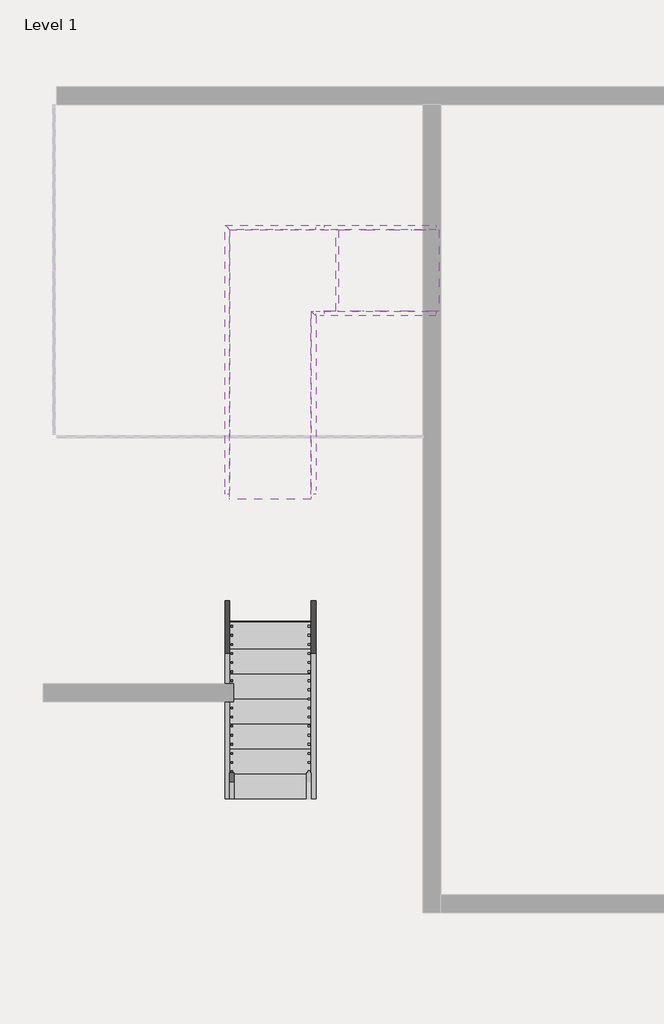
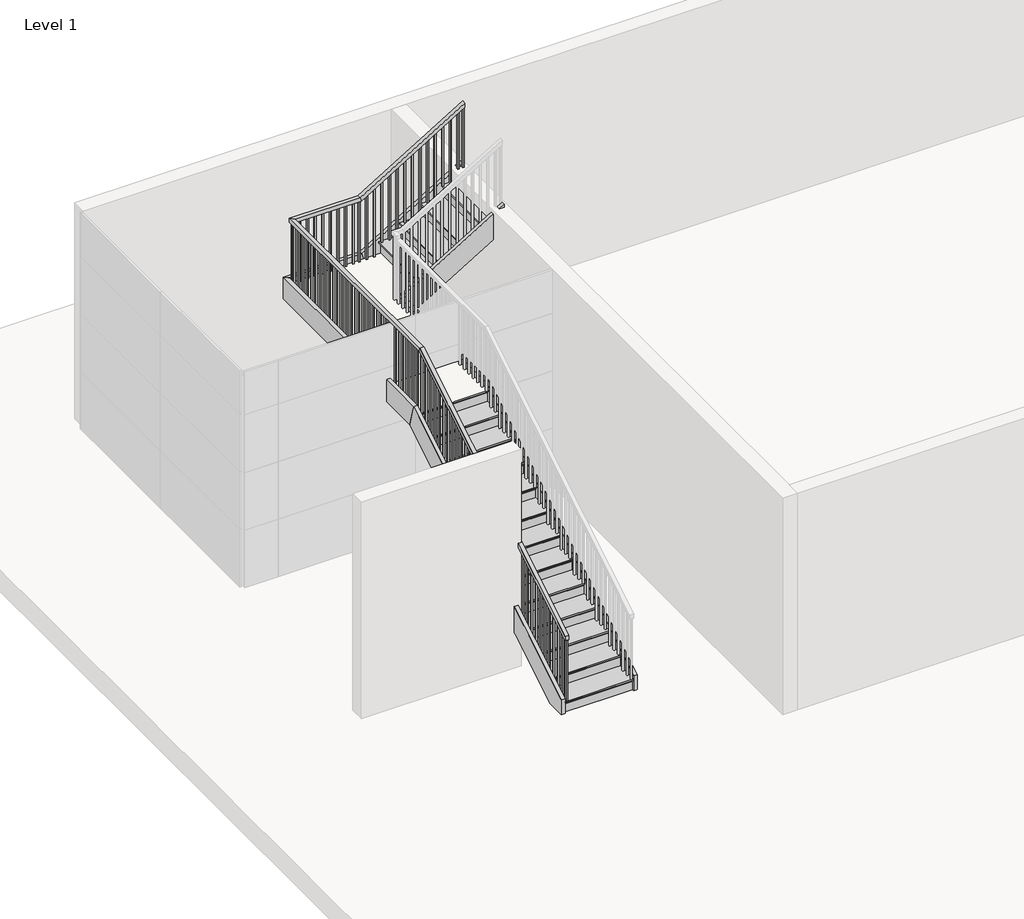
# One storey, part 2 of 2: 8 members, 2 stair flights, 1 railing, 1 slab.
"""IFC4 building model written with IfcOpenShell, lengths in millimetres."""

from ifc_helpers import new_model, si_unit, frame, origin, place, context, project, spatial, polyline, outline, extrude, faceted_brep, transform, mapped, element, save
from components import non_monolithic_landing_d9f9278d, stair_flight_de60d348, stair_flight_1517cfd2

model = new_model("IFC4")

# Units and contexts
model_context = context("Model", 3, world=origin())
ifc_project = project(units=[si_unit("LENGTHUNIT", "METRE", prefix="MILLI")], contexts=[model_context])

# Site, building, storey
site = spatial("IfcSite", under=ifc_project)
building = spatial("IfcBuilding", under=site)
storey = spatial("IfcBuildingStorey", under=building, Name="Level 1", Elevation=0.0)

# Members
placement = place(None, origin())
element("IfcMember", 1, ObjectType="Stringer - 2\" Width", at=placement, inside=storey, context=model_context, shape_type="SweptSolid", body=[
    extrude(outline(polyline([(1898.2635177, 0.0), (1898.2635177, 212.114512), (5306.204573, 2277.5333333), (5391.3590295, 1972.7333333), (2136.3490295, 0.0), (1898.2635177, 0.0)])), frame((-9085.0823175, 0.0, 0.0), z_axis=(1.0, 0.0, 0.0), x_axis=(0.0, 1.0, 0.0)), (0.0, 0.0, 1.0), 50.8),
])
element("IfcMember", 2, ObjectType="Stringer - 2\" Width", at=placement, inside=storey, context=model_context, shape_type="SweptSolid", body=[
    extrude(outline(polyline([(1898.2635177, 0.0), (1898.2635177, 212.114512), (5306.204573, 2277.5333333), (5391.3590295, 1972.7333333), (2136.3490295, 0.0), (1898.2635177, 0.0)])), frame((-8119.8823175, 0.0, 0.0), z_axis=(1.0, 0.0, 0.0), x_axis=(0.0, 1.0, 0.0)), (0.0, 0.0, 1.0), 50.8),
])
element("IfcMember", 3, ObjectType="Stringer - 2\" Width", at=placement, inside=storey, context=model_context, shape_type="SweptSolid", body=[
    extrude(outline(polyline([(2277.5333333, -8064.7412622), (1972.7333333, -7979.5868057), (2734.3724171, -6722.8823175), (3090.7811786, -6722.8823175), (2277.5333333, -8064.7412622)])), frame((0.0, 8266.605876, 0.0), z_axis=(0.0, 1.0, 0.0), x_axis=(0.0, 0.0, 1.0)), (0.0, 0.0, 1.0), 50.8),
])
element("IfcMember", 4, ObjectType="Stringer - 2\" Width", at=placement, inside=storey, context=model_context, shape_type="SweptSolid", body=[
    extrude(outline(polyline([(2277.5333333, -8064.7412622), (1972.7333333, -7979.5868057), (2734.3724171, -6722.8823175), (3090.7811786, -6722.8823175), (2277.5333333, -8064.7412622)])), frame((0.0, 7301.405876, 0.0), z_axis=(0.0, 1.0, 0.0), x_axis=(0.0, 0.0, 1.0)), (0.0, 0.0, 1.0), 50.8),
])
element("IfcMember", 5, ObjectType="Stringer - 2\" Width", at=placement, inside=storey, context=model_context, shape_type="Brep", body=[
    faceted_brep([(-8064.7412622, 8266.605876, 2277.5333333), (-8064.7412622, 8317.405876, 2277.5333333), (-9085.0823175, 8317.405876, 2277.5333333), (-9034.2823175, 8266.605876, 2277.5333333), (-7979.5868057, 8266.605876, 1972.7333333), (-9034.2823175, 8266.605876, 1972.7333333), (-7979.5868057, 8317.405876, 1972.7333333), (-9085.0823175, 8317.405876, 1972.7333333)], [[[0, 1, 2, 3]], [[4, 0, 3, 5]], [[6, 4, 5, 7]], [[1, 6, 7, 2]], [[1, 0, 4, 6]], [[2, 7, 5, 3]]]),
])
element("IfcMember", 6, ObjectType="Stringer - 2\" Width", at=placement, inside=storey, context=model_context, shape_type="Brep", body=[
    faceted_brep([(-9034.2823175, 8266.605876, 2277.5333333), (-9085.0823175, 8317.405876, 2277.5333333), (-9085.0823175, 5306.204573, 2277.5333333), (-9034.2823175, 5306.204573, 2277.5333333), (-9034.2823175, 8266.605876, 1972.7333333), (-9034.2823175, 5391.3590295, 1972.7333333), (-9085.0823175, 8317.405876, 1972.7333333), (-9085.0823175, 5391.3590295, 1972.7333333)], [[[0, 1, 2, 3]], [[4, 0, 3, 5]], [[6, 4, 5, 7]], [[1, 6, 7, 2]], [[1, 0, 4, 6]], [[2, 7, 5, 3]]]),
])
element("IfcMember", 7, ObjectType="Stringer - 2\" Width", at=placement, inside=storey, context=model_context, shape_type="Brep", body=[
    faceted_brep([(-8119.8823175, 5306.204573, 2277.5333333), (-8069.0823175, 5306.204573, 2277.5333333), (-8069.0823175, 7301.405876, 2277.5333333), (-8119.8823175, 7352.205876, 2277.5333333), (-8119.8823175, 5391.3590295, 1972.7333333), (-8119.8823175, 7352.205876, 1972.7333333), (-8069.0823175, 5391.3590295, 1972.7333333), (-8069.0823175, 7301.405876, 1972.7333333)], [[[0, 1, 2, 3]], [[4, 0, 3, 5]], [[6, 4, 5, 7]], [[1, 6, 7, 2]], [[1, 0, 4, 6]], [[2, 7, 5, 3]]]),
])
element("IfcMember", 8, ObjectType="Stringer - 2\" Width", at=placement, inside=storey, context=model_context, shape_type="Brep", body=[
    faceted_brep([(-8119.8823175, 7352.205876, 2277.5333333), (-8069.0823175, 7301.405876, 2277.5333333), (-8064.7412622, 7301.405876, 2277.5333333), (-8064.7412622, 7352.205876, 2277.5333333), (-8119.8823175, 7352.205876, 1972.7333333), (-7979.5868057, 7352.205876, 1972.7333333), (-8069.0823175, 7301.405876, 1972.7333333), (-7979.5868057, 7301.405876, 1972.7333333)], [[[0, 1, 2, 3]], [[4, 0, 3, 5]], [[6, 4, 5, 7]], [[1, 6, 7, 2]], [[1, 0, 4, 6]], [[2, 7, 5, 3]]]),
])

# Railing
element("IfcRailing", 9, ObjectType="Handrail - Rectangular", at=placement, inside=storey, context=model_context, shape_type="SolidModel", body=[
    faceted_brep([(-9034.2823175, 1898.2635177, 1083.7333333), (-9034.2823175, 1898.2635177, 1024.3318731), (-8983.4823175, 1898.2635177, 1024.3318731), (-8983.4823175, 1898.2635177, 1083.7333333), (-9034.2823175, 5251.0635177, 3115.7333333), (-9034.2823175, 5265.2559271, 3064.9333333), (-8983.4823175, 5265.2559271, 3064.9333333), (-8983.4823175, 5251.0635177, 3115.7333333), (-9034.2823175, 8266.605876, 3115.7333333), (-9034.2823175, 8266.605876, 3064.9333333), (-8983.4823175, 8215.805876, 3064.9333333), (-8983.4823175, 8215.805876, 3115.7333333), (-8119.8823175, 8266.605876, 3115.7333333), (-8105.6899081, 8266.605876, 3064.9333333), (-8105.6899081, 8215.805876, 3064.9333333), (-8119.8823175, 8215.805876, 3115.7333333), (-6722.8823175, 8266.605876, 3962.4), (-6722.8823175, 8215.805876, 3962.4), (-6722.8823175, 8215.805876, 3902.9985397), (-6722.8823175, 8266.605876, 3902.9985397)], [[[0, 1, 2, 3]], [[1, 0, 4, 5]], [[2, 1, 5, 6]], [[3, 2, 6, 7]], [[0, 3, 7, 4]], [[5, 4, 8, 9]], [[6, 5, 9, 10]], [[7, 6, 10, 11]], [[4, 7, 11, 8]], [[9, 8, 12, 13]], [[10, 9, 13, 14]], [[11, 10, 14, 15]], [[8, 11, 15, 12]], [[16, 17, 18, 19]], [[13, 12, 16, 19]], [[14, 13, 19, 18]], [[15, 14, 18, 17]], [[12, 15, 17, 16]]]),
    extrude(outline(polyline([(3851.0439943, -6808.6073175), (2878.6666667, -6808.6073175), (2878.6666667, -6789.5573175), (3862.5894488, -6789.5573175), (3851.0439943, -6808.6073175)])), frame((0.0, 8231.680876, 0.0), z_axis=(0.0, 1.0, 0.0), x_axis=(0.0, 0.0, 1.0)), (0.0, 0.0, 1.0), 19.05),
    extrude(outline(polyline([(3789.4682367, -6910.2073175), (2878.6666667, -6910.2073175), (2878.6666667, -6891.1573175), (3801.0136913, -6891.1573175), (3789.4682367, -6910.2073175)])), frame((0.0, 8231.680876, 0.0), z_axis=(0.0, 1.0, 0.0), x_axis=(0.0, 0.0, 1.0)), (0.0, 0.0, 1.0), 19.05),
    extrude(outline(polyline([(3727.8924791, -7011.8073175), (2878.6666667, -7011.8073175), (2878.6666667, -6992.7573175), (3739.4379337, -6992.7573175), (3727.8924791, -7011.8073175)])), frame((0.0, 8231.680876, 0.0), z_axis=(0.0, 1.0, 0.0), x_axis=(0.0, 0.0, 1.0)), (0.0, 0.0, 1.0), 19.05),
    extrude(outline(polyline([(3666.3167216, -7113.4073175), (2709.3333333, -7113.4073175), (2709.3333333, -7094.3573175), (3677.8621761, -7094.3573175), (3666.3167216, -7113.4073175)])), frame((0.0, 8231.680876, 0.0), z_axis=(0.0, 1.0, 0.0), x_axis=(0.0, 0.0, 1.0)), (0.0, 0.0, 1.0), 19.05),
    extrude(outline(polyline([(3604.740964, -7215.0073175), (2709.3333333, -7215.0073175), (2709.3333333, -7195.9573175), (3616.2864185, -7195.9573175), (3604.740964, -7215.0073175)])), frame((0.0, 8231.680876, 0.0), z_axis=(0.0, 1.0, 0.0), x_axis=(0.0, 0.0, 1.0)), (0.0, 0.0, 1.0), 19.05),
    extrude(outline(polyline([(3543.1652064, -7316.6073175), (2540.0, -7316.6073175), (2540.0, -7297.5573175), (3554.710661, -7297.5573175), (3543.1652064, -7316.6073175)])), frame((0.0, 8231.680876, 0.0), z_axis=(0.0, 1.0, 0.0), x_axis=(0.0, 0.0, 1.0)), (0.0, 0.0, 1.0), 19.05),
    extrude(outline(polyline([(3481.5894488, -7418.2073175), (2540.0, -7418.2073175), (2540.0, -7399.1573175), (3493.1349034, -7399.1573175), (3481.5894488, -7418.2073175)])), frame((0.0, 8231.680876, 0.0), z_axis=(0.0, 1.0, 0.0), x_axis=(0.0, 0.0, 1.0)), (0.0, 0.0, 1.0), 19.05),
    extrude(outline(polyline([(3420.0136913, -7519.8073175), (2540.0, -7519.8073175), (2540.0, -7500.7573175), (3431.5591458, -7500.7573175), (3420.0136913, -7519.8073175)])), frame((0.0, 8231.680876, 0.0), z_axis=(0.0, 1.0, 0.0), x_axis=(0.0, 0.0, 1.0)), (0.0, 0.0, 1.0), 19.05),
    extrude(outline(polyline([(3358.4379337, -7621.4073175), (2370.6666667, -7621.4073175), (2370.6666667, -7602.3573175), (3369.9833882, -7602.3573175), (3358.4379337, -7621.4073175)])), frame((0.0, 8231.680876, 0.0), z_axis=(0.0, 1.0, 0.0), x_axis=(0.0, 0.0, 1.0)), (0.0, 0.0, 1.0), 19.05),
    extrude(outline(polyline([(3296.8621761, -7723.0073175), (2370.6666667, -7723.0073175), (2370.6666667, -7703.9573175), (3308.4076307, -7703.9573175), (3296.8621761, -7723.0073175)])), frame((0.0, 8231.680876, 0.0), z_axis=(0.0, 1.0, 0.0), x_axis=(0.0, 0.0, 1.0)), (0.0, 0.0, 1.0), 19.05),
    extrude(outline(polyline([(3235.2864185, -7824.6073175), (2370.6666667, -7824.6073175), (2370.6666667, -7805.5573175), (3246.8318731, -7805.5573175), (3235.2864185, -7824.6073175)])), frame((0.0, 8231.680876, 0.0), z_axis=(0.0, 1.0, 0.0), x_axis=(0.0, 0.0, 1.0)), (0.0, 0.0, 1.0), 19.05),
    extrude(outline(polyline([(3173.710661, -7926.2073175), (2201.3333333, -7926.2073175), (2201.3333333, -7907.1573175), (3185.2561155, -7907.1573175), (3173.710661, -7926.2073175)])), frame((0.0, 8231.680876, 0.0), z_axis=(0.0, 1.0, 0.0), x_axis=(0.0, 0.0, 1.0)), (0.0, 0.0, 1.0), 19.05),
    extrude(outline(polyline([(3112.1349034, -8027.8073175), (2201.3333333, -8027.8073175), (2201.3333333, -8008.7573175), (3123.6803579, -8008.7573175), (3112.1349034, -8027.8073175)])), frame((0.0, 8231.680876, 0.0), z_axis=(0.0, 1.0, 0.0), x_axis=(0.0, 0.0, 1.0)), (0.0, 0.0, 1.0), 19.05),
    extrude(outline(polyline([(-8205.6073175, 8250.730876), (-8186.5573175, 8250.730876), (-8186.5573175, 8231.680876), (-8205.6073175, 8231.680876), (-8205.6073175, 8250.730876)])), frame((0.0, 0.0, 2201.3333333), z_axis=(0.0, 0.0, 1.0), x_axis=(1.0, 0.0, 0.0)), (0.0, 0.0, 1.0), 863.6),
    extrude(outline(polyline([(-8307.2073175, 8250.730876), (-8288.1573175, 8250.730876), (-8288.1573175, 8231.680876), (-8307.2073175, 8231.680876), (-8307.2073175, 8250.730876)])), frame((0.0, 0.0, 2201.3333333), z_axis=(0.0, 0.0, 1.0), x_axis=(1.0, 0.0, 0.0)), (0.0, 0.0, 1.0), 863.6),
    extrude(outline(polyline([(-8408.8073175, 8250.730876), (-8389.7573175, 8250.730876), (-8389.7573175, 8231.680876), (-8408.8073175, 8231.680876), (-8408.8073175, 8250.730876)])), frame((0.0, 0.0, 2201.3333333), z_axis=(0.0, 0.0, 1.0), x_axis=(1.0, 0.0, 0.0)), (0.0, 0.0, 1.0), 863.6),
    extrude(outline(polyline([(-8510.4073175, 8250.730876), (-8491.3573175, 8250.730876), (-8491.3573175, 8231.680876), (-8510.4073175, 8231.680876), (-8510.4073175, 8250.730876)])), frame((0.0, 0.0, 2201.3333333), z_axis=(0.0, 0.0, 1.0), x_axis=(1.0, 0.0, 0.0)), (0.0, 0.0, 1.0), 863.6),
    extrude(outline(polyline([(-8612.0073175, 8250.730876), (-8592.9573175, 8250.730876), (-8592.9573175, 8231.680876), (-8612.0073175, 8231.680876), (-8612.0073175, 8250.730876)])), frame((0.0, 0.0, 2201.3333333), z_axis=(0.0, 0.0, 1.0), x_axis=(1.0, 0.0, 0.0)), (0.0, 0.0, 1.0), 863.6),
    extrude(outline(polyline([(-8713.6073175, 8250.730876), (-8694.5573175, 8250.730876), (-8694.5573175, 8231.680876), (-8713.6073175, 8231.680876), (-8713.6073175, 8250.730876)])), frame((0.0, 0.0, 2201.3333333), z_axis=(0.0, 0.0, 1.0), x_axis=(1.0, 0.0, 0.0)), (0.0, 0.0, 1.0), 863.6),
    extrude(outline(polyline([(-8815.2073175, 8250.730876), (-8796.1573175, 8250.730876), (-8796.1573175, 8231.680876), (-8815.2073175, 8231.680876), (-8815.2073175, 8250.730876)])), frame((0.0, 0.0, 2201.3333333), z_axis=(0.0, 0.0, 1.0), x_axis=(1.0, 0.0, 0.0)), (0.0, 0.0, 1.0), 863.6),
    extrude(outline(polyline([(-8916.8073175, 8250.730876), (-8897.7573175, 8250.730876), (-8897.7573175, 8231.680876), (-8916.8073175, 8231.680876), (-8916.8073175, 8250.730876)])), frame((0.0, 0.0, 2201.3333333), z_axis=(0.0, 0.0, 1.0), x_axis=(1.0, 0.0, 0.0)), (0.0, 0.0, 1.0), 863.6),
    extrude(outline(polyline([(-9018.4073175, 8187.9385177), (-9018.4073175, 8206.9885177), (-8999.3573175, 8206.9885177), (-8999.3573175, 8187.9385177), (-9018.4073175, 8187.9385177)])), frame((0.0, 0.0, 2201.3333333), z_axis=(0.0, 0.0, 1.0), x_axis=(1.0, 0.0, 0.0)), (0.0, 0.0, 1.0), 863.6),
    extrude(outline(polyline([(-9018.4073175, 8086.3385177), (-9018.4073175, 8105.3885177), (-8999.3573175, 8105.3885177), (-8999.3573175, 8086.3385177), (-9018.4073175, 8086.3385177)])), frame((0.0, 0.0, 2201.3333333), z_axis=(0.0, 0.0, 1.0), x_axis=(1.0, 0.0, 0.0)), (0.0, 0.0, 1.0), 863.6),
    extrude(outline(polyline([(-9018.4073175, 7984.7385177), (-9018.4073175, 8003.7885177), (-8999.3573175, 8003.7885177), (-8999.3573175, 7984.7385177), (-9018.4073175, 7984.7385177)])), frame((0.0, 0.0, 2201.3333333), z_axis=(0.0, 0.0, 1.0), x_axis=(1.0, 0.0, 0.0)), (0.0, 0.0, 1.0), 863.6),
    extrude(outline(polyline([(-9018.4073175, 7883.1385177), (-9018.4073175, 7902.1885177), (-8999.3573175, 7902.1885177), (-8999.3573175, 7883.1385177), (-9018.4073175, 7883.1385177)])), frame((0.0, 0.0, 2201.3333333), z_axis=(0.0, 0.0, 1.0), x_axis=(1.0, 0.0, 0.0)), (0.0, 0.0, 1.0), 863.6),
    extrude(outline(polyline([(-9018.4073175, 7781.5385177), (-9018.4073175, 7800.5885177), (-8999.3573175, 7800.5885177), (-8999.3573175, 7781.5385177), (-9018.4073175, 7781.5385177)])), frame((0.0, 0.0, 2201.3333333), z_axis=(0.0, 0.0, 1.0), x_axis=(1.0, 0.0, 0.0)), (0.0, 0.0, 1.0), 863.6),
    extrude(outline(polyline([(-9018.4073175, 7679.9385177), (-9018.4073175, 7698.9885177), (-8999.3573175, 7698.9885177), (-8999.3573175, 7679.9385177), (-9018.4073175, 7679.9385177)])), frame((0.0, 0.0, 2201.3333333), z_axis=(0.0, 0.0, 1.0), x_axis=(1.0, 0.0, 0.0)), (0.0, 0.0, 1.0), 863.6),
    extrude(outline(polyline([(-9018.4073175, 7578.3385177), (-9018.4073175, 7597.3885177), (-8999.3573175, 7597.3885177), (-8999.3573175, 7578.3385177), (-9018.4073175, 7578.3385177)])), frame((0.0, 0.0, 2201.3333333), z_axis=(0.0, 0.0, 1.0), x_axis=(1.0, 0.0, 0.0)), (0.0, 0.0, 1.0), 863.6),
    extrude(outline(polyline([(-9018.4073175, 7476.7385177), (-9018.4073175, 7495.7885177), (-8999.3573175, 7495.7885177), (-8999.3573175, 7476.7385177), (-9018.4073175, 7476.7385177)])), frame((0.0, 0.0, 2201.3333333), z_axis=(0.0, 0.0, 1.0), x_axis=(1.0, 0.0, 0.0)), (0.0, 0.0, 1.0), 863.6),
    extrude(outline(polyline([(-9018.4073175, 7375.1385177), (-9018.4073175, 7394.1885177), (-8999.3573175, 7394.1885177), (-8999.3573175, 7375.1385177), (-9018.4073175, 7375.1385177)])), frame((0.0, 0.0, 2201.3333333), z_axis=(0.0, 0.0, 1.0), x_axis=(1.0, 0.0, 0.0)), (0.0, 0.0, 1.0), 863.6),
    extrude(outline(polyline([(-9018.4073175, 7273.5385177), (-9018.4073175, 7292.5885177), (-8999.3573175, 7292.5885177), (-8999.3573175, 7273.5385177), (-9018.4073175, 7273.5385177)])), frame((0.0, 0.0, 2201.3333333), z_axis=(0.0, 0.0, 1.0), x_axis=(1.0, 0.0, 0.0)), (0.0, 0.0, 1.0), 863.6),
    extrude(outline(polyline([(-9018.4073175, 7171.9385177), (-9018.4073175, 7190.9885177), (-8999.3573175, 7190.9885177), (-8999.3573175, 7171.9385177), (-9018.4073175, 7171.9385177)])), frame((0.0, 0.0, 2201.3333333), z_axis=(0.0, 0.0, 1.0), x_axis=(1.0, 0.0, 0.0)), (0.0, 0.0, 1.0), 863.6),
    extrude(outline(polyline([(-9018.4073175, 7070.3385177), (-9018.4073175, 7089.3885177), (-8999.3573175, 7089.3885177), (-8999.3573175, 7070.3385177), (-9018.4073175, 7070.3385177)])), frame((0.0, 0.0, 2201.3333333), z_axis=(0.0, 0.0, 1.0), x_axis=(1.0, 0.0, 0.0)), (0.0, 0.0, 1.0), 863.6),
    extrude(outline(polyline([(-9018.4073175, 6968.7385177), (-9018.4073175, 6987.7885177), (-8999.3573175, 6987.7885177), (-8999.3573175, 6968.7385177), (-9018.4073175, 6968.7385177)])), frame((0.0, 0.0, 2201.3333333), z_axis=(0.0, 0.0, 1.0), x_axis=(1.0, 0.0, 0.0)), (0.0, 0.0, 1.0), 863.6),
    extrude(outline(polyline([(-9018.4073175, 6867.1385177), (-9018.4073175, 6886.1885177), (-8999.3573175, 6886.1885177), (-8999.3573175, 6867.1385177), (-9018.4073175, 6867.1385177)])), frame((0.0, 0.0, 2201.3333333), z_axis=(0.0, 0.0, 1.0), x_axis=(1.0, 0.0, 0.0)), (0.0, 0.0, 1.0), 863.6),
    extrude(outline(polyline([(-9018.4073175, 6765.5385177), (-9018.4073175, 6784.5885177), (-8999.3573175, 6784.5885177), (-8999.3573175, 6765.5385177), (-9018.4073175, 6765.5385177)])), frame((0.0, 0.0, 2201.3333333), z_axis=(0.0, 0.0, 1.0), x_axis=(1.0, 0.0, 0.0)), (0.0, 0.0, 1.0), 863.6),
    extrude(outline(polyline([(-9018.4073175, 6663.9385177), (-9018.4073175, 6682.9885177), (-8999.3573175, 6682.9885177), (-8999.3573175, 6663.9385177), (-9018.4073175, 6663.9385177)])), frame((0.0, 0.0, 2201.3333333), z_axis=(0.0, 0.0, 1.0), x_axis=(1.0, 0.0, 0.0)), (0.0, 0.0, 1.0), 863.6),
    extrude(outline(polyline([(-9018.4073175, 6562.3385177), (-9018.4073175, 6581.3885177), (-8999.3573175, 6581.3885177), (-8999.3573175, 6562.3385177), (-9018.4073175, 6562.3385177)])), frame((0.0, 0.0, 2201.3333333), z_axis=(0.0, 0.0, 1.0), x_axis=(1.0, 0.0, 0.0)), (0.0, 0.0, 1.0), 863.6),
    extrude(outline(polyline([(-9018.4073175, 6460.7385177), (-9018.4073175, 6479.7885177), (-8999.3573175, 6479.7885177), (-8999.3573175, 6460.7385177), (-9018.4073175, 6460.7385177)])), frame((0.0, 0.0, 2201.3333333), z_axis=(0.0, 0.0, 1.0), x_axis=(1.0, 0.0, 0.0)), (0.0, 0.0, 1.0), 863.6),
    extrude(outline(polyline([(-9018.4073175, 6359.1385177), (-9018.4073175, 6378.1885177), (-8999.3573175, 6378.1885177), (-8999.3573175, 6359.1385177), (-9018.4073175, 6359.1385177)])), frame((0.0, 0.0, 2201.3333333), z_axis=(0.0, 0.0, 1.0), x_axis=(1.0, 0.0, 0.0)), (0.0, 0.0, 1.0), 863.6),
    extrude(outline(polyline([(-9018.4073175, 6257.5385177), (-9018.4073175, 6276.5885177), (-8999.3573175, 6276.5885177), (-8999.3573175, 6257.5385177), (-9018.4073175, 6257.5385177)])), frame((0.0, 0.0, 2201.3333333), z_axis=(0.0, 0.0, 1.0), x_axis=(1.0, 0.0, 0.0)), (0.0, 0.0, 1.0), 863.6),
    extrude(outline(polyline([(-9018.4073175, 6155.9385177), (-9018.4073175, 6174.9885177), (-8999.3573175, 6174.9885177), (-8999.3573175, 6155.9385177), (-9018.4073175, 6155.9385177)])), frame((0.0, 0.0, 2201.3333333), z_axis=(0.0, 0.0, 1.0), x_axis=(1.0, 0.0, 0.0)), (0.0, 0.0, 1.0), 863.6),
    extrude(outline(polyline([(-9018.4073175, 6054.3385177), (-9018.4073175, 6073.3885177), (-8999.3573175, 6073.3885177), (-8999.3573175, 6054.3385177), (-9018.4073175, 6054.3385177)])), frame((0.0, 0.0, 2201.3333333), z_axis=(0.0, 0.0, 1.0), x_axis=(1.0, 0.0, 0.0)), (0.0, 0.0, 1.0), 863.6),
    extrude(outline(polyline([(-9018.4073175, 5952.7385177), (-9018.4073175, 5971.7885177), (-8999.3573175, 5971.7885177), (-8999.3573175, 5952.7385177), (-9018.4073175, 5952.7385177)])), frame((0.0, 0.0, 2201.3333333), z_axis=(0.0, 0.0, 1.0), x_axis=(1.0, 0.0, 0.0)), (0.0, 0.0, 1.0), 863.6),
    extrude(outline(polyline([(-9018.4073175, 5851.1385177), (-9018.4073175, 5870.1885177), (-8999.3573175, 5870.1885177), (-8999.3573175, 5851.1385177), (-9018.4073175, 5851.1385177)])), frame((0.0, 0.0, 2201.3333333), z_axis=(0.0, 0.0, 1.0), x_axis=(1.0, 0.0, 0.0)), (0.0, 0.0, 1.0), 863.6),
    extrude(outline(polyline([(-9018.4073175, 5749.5385177), (-9018.4073175, 5768.5885177), (-8999.3573175, 5768.5885177), (-8999.3573175, 5749.5385177), (-9018.4073175, 5749.5385177)])), frame((0.0, 0.0, 2201.3333333), z_axis=(0.0, 0.0, 1.0), x_axis=(1.0, 0.0, 0.0)), (0.0, 0.0, 1.0), 863.6),
    extrude(outline(polyline([(-9018.4073175, 5647.9385177), (-9018.4073175, 5666.9885177), (-8999.3573175, 5666.9885177), (-8999.3573175, 5647.9385177), (-9018.4073175, 5647.9385177)])), frame((0.0, 0.0, 2201.3333333), z_axis=(0.0, 0.0, 1.0), x_axis=(1.0, 0.0, 0.0)), (0.0, 0.0, 1.0), 863.6),
    extrude(outline(polyline([(-9018.4073175, 5546.3385177), (-9018.4073175, 5565.3885177), (-8999.3573175, 5565.3885177), (-8999.3573175, 5546.3385177), (-9018.4073175, 5546.3385177)])), frame((0.0, 0.0, 2201.3333333), z_axis=(0.0, 0.0, 1.0), x_axis=(1.0, 0.0, 0.0)), (0.0, 0.0, 1.0), 863.6),
    extrude(outline(polyline([(-9018.4073175, 5444.7385177), (-9018.4073175, 5463.7885177), (-8999.3573175, 5463.7885177), (-8999.3573175, 5444.7385177), (-9018.4073175, 5444.7385177)])), frame((0.0, 0.0, 2201.3333333), z_axis=(0.0, 0.0, 1.0), x_axis=(1.0, 0.0, 0.0)), (0.0, 0.0, 1.0), 863.6),
    extrude(outline(polyline([(-9018.4073175, 5343.1385177), (-9018.4073175, 5362.1885177), (-8999.3573175, 5362.1885177), (-8999.3573175, 5343.1385177), (-9018.4073175, 5343.1385177)])), frame((0.0, 0.0, 2201.3333333), z_axis=(0.0, 0.0, 1.0), x_axis=(1.0, 0.0, 0.0)), (0.0, 0.0, 1.0), 863.6),
    extrude(outline(polyline([(5158.9885177, 3000.5288428), (5158.9885177, 2032.0), (5139.9385177, 2032.0), (5139.9385177, 2988.9833882), (5158.9885177, 3000.5288428)])), frame((-9018.4073175, 0.0, 0.0), z_axis=(1.0, 0.0, 0.0), x_axis=(0.0, 1.0, 0.0)), (0.0, 0.0, 1.0), 19.05),
    extrude(outline(polyline([(5057.3885177, 2938.9530852), (5057.3885177, 2032.0), (5038.3385177, 2032.0), (5038.3385177, 2927.4076307), (5057.3885177, 2938.9530852)])), frame((-9018.4073175, 0.0, 0.0), z_axis=(1.0, 0.0, 0.0), x_axis=(0.0, 1.0, 0.0)), (0.0, 0.0, 1.0), 19.05),
    extrude(outline(polyline([(4955.7885177, 2877.3773276), (4955.7885177, 1862.6666667), (4936.7385177, 1862.6666667), (4936.7385177, 2865.8318731), (4955.7885177, 2877.3773276)])), frame((-9018.4073175, 0.0, 0.0), z_axis=(1.0, 0.0, 0.0), x_axis=(0.0, 1.0, 0.0)), (0.0, 0.0, 1.0), 19.05),
    extrude(outline(polyline([(4854.1885177, 2815.80157), (4854.1885177, 1862.6666667), (4835.1385177, 1862.6666667), (4835.1385177, 2804.2561155), (4854.1885177, 2815.80157)])), frame((-9018.4073175, 0.0, 0.0), z_axis=(1.0, 0.0, 0.0), x_axis=(0.0, 1.0, 0.0)), (0.0, 0.0, 1.0), 19.05),
    extrude(outline(polyline([(4752.5885177, 2754.2258125), (4752.5885177, 1862.6666667), (4733.5385177, 1862.6666667), (4733.5385177, 2742.6803579), (4752.5885177, 2754.2258125)])), frame((-9018.4073175, 0.0, 0.0), z_axis=(1.0, 0.0, 0.0), x_axis=(0.0, 1.0, 0.0)), (0.0, 0.0, 1.0), 19.05),
    extrude(outline(polyline([(4650.9885177, 2692.6500549), (4650.9885177, 1693.3333333), (4631.9385177, 1693.3333333), (4631.9385177, 2681.1046004), (4650.9885177, 2692.6500549)])), frame((-9018.4073175, 0.0, 0.0), z_axis=(1.0, 0.0, 0.0), x_axis=(0.0, 1.0, 0.0)), (0.0, 0.0, 1.0), 19.05),
    extrude(outline(polyline([(4549.3885177, 2631.0742973), (4549.3885177, 1693.3333333), (4530.3385177, 1693.3333333), (4530.3385177, 2619.5288428), (4549.3885177, 2631.0742973)])), frame((-9018.4073175, 0.0, 0.0), z_axis=(1.0, 0.0, 0.0), x_axis=(0.0, 1.0, 0.0)), (0.0, 0.0, 1.0), 19.05),
    extrude(outline(polyline([(4447.7885177, 2569.4985397), (4447.7885177, 1693.3333333), (4428.7385177, 1693.3333333), (4428.7385177, 2557.9530852), (4447.7885177, 2569.4985397)])), frame((-9018.4073175, 0.0, 0.0), z_axis=(1.0, 0.0, 0.0), x_axis=(0.0, 1.0, 0.0)), (0.0, 0.0, 1.0), 19.05),
    extrude(outline(polyline([(4346.1885177, 2507.9227822), (4346.1885177, 1524.0), (4327.1385177, 1524.0), (4327.1385177, 2496.3773276), (4346.1885177, 2507.9227822)])), frame((-9018.4073175, 0.0, 0.0), z_axis=(1.0, 0.0, 0.0), x_axis=(0.0, 1.0, 0.0)), (0.0, 0.0, 1.0), 19.05),
    extrude(outline(polyline([(4244.5885177, 2446.3470246), (4244.5885177, 1524.0), (4225.5385177, 1524.0), (4225.5385177, 2434.80157), (4244.5885177, 2446.3470246)])), frame((-9018.4073175, 0.0, 0.0), z_axis=(1.0, 0.0, 0.0), x_axis=(0.0, 1.0, 0.0)), (0.0, 0.0, 1.0), 19.05),
    extrude(outline(polyline([(4142.9885177, 2384.771267), (4142.9885177, 1524.0), (4123.9385177, 1524.0), (4123.9385177, 2373.2258125), (4142.9885177, 2384.771267)])), frame((-9018.4073175, 0.0, 0.0), z_axis=(1.0, 0.0, 0.0), x_axis=(0.0, 1.0, 0.0)), (0.0, 0.0, 1.0), 19.05),
    extrude(outline(polyline([(4041.3885177, 2323.1955094), (4041.3885177, 1354.6666667), (4022.3385177, 1354.6666667), (4022.3385177, 2311.6500549), (4041.3885177, 2323.1955094)])), frame((-9018.4073175, 0.0, 0.0), z_axis=(1.0, 0.0, 0.0), x_axis=(0.0, 1.0, 0.0)), (0.0, 0.0, 1.0), 19.05),
    extrude(outline(polyline([(3939.7885177, 2261.6197519), (3939.7885177, 1354.6666667), (3920.7385177, 1354.6666667), (3920.7385177, 2250.0742973), (3939.7885177, 2261.6197519)])), frame((-9018.4073175, 0.0, 0.0), z_axis=(1.0, 0.0, 0.0), x_axis=(0.0, 1.0, 0.0)), (0.0, 0.0, 1.0), 19.05),
    extrude(outline(polyline([(3838.1885177, 2200.0439943), (3838.1885177, 1185.3333333), (3819.1385177, 1185.3333333), (3819.1385177, 2188.4985397), (3838.1885177, 2200.0439943)])), frame((-9018.4073175, 0.0, 0.0), z_axis=(1.0, 0.0, 0.0), x_axis=(0.0, 1.0, 0.0)), (0.0, 0.0, 1.0), 19.05),
    extrude(outline(polyline([(3736.5885177, 2138.4682367), (3736.5885177, 1185.3333333), (3717.5385177, 1185.3333333), (3717.5385177, 2126.9227822), (3736.5885177, 2138.4682367)])), frame((-9018.4073175, 0.0, 0.0), z_axis=(1.0, 0.0, 0.0), x_axis=(0.0, 1.0, 0.0)), (0.0, 0.0, 1.0), 19.05),
    extrude(outline(polyline([(3634.9885177, 2076.8924791), (3634.9885177, 1185.3333333), (3615.9385177, 1185.3333333), (3615.9385177, 2065.3470246), (3634.9885177, 2076.8924791)])), frame((-9018.4073175, 0.0, 0.0), z_axis=(1.0, 0.0, 0.0), x_axis=(0.0, 1.0, 0.0)), (0.0, 0.0, 1.0), 19.05),
    extrude(outline(polyline([(3533.3885177, 2015.3167216), (3533.3885177, 1016.0), (3514.3385177, 1016.0), (3514.3385177, 2003.771267), (3533.3885177, 2015.3167216)])), frame((-9018.4073175, 0.0, 0.0), z_axis=(1.0, 0.0, 0.0), x_axis=(0.0, 1.0, 0.0)), (0.0, 0.0, 1.0), 19.05),
    extrude(outline(polyline([(3431.7885177, 1953.740964), (3431.7885177, 1016.0), (3412.7385177, 1016.0), (3412.7385177, 1942.1955094), (3431.7885177, 1953.740964)])), frame((-9018.4073175, 0.0, 0.0), z_axis=(1.0, 0.0, 0.0), x_axis=(0.0, 1.0, 0.0)), (0.0, 0.0, 1.0), 19.05),
    extrude(outline(polyline([(3330.1885177, 1892.1652064), (3330.1885177, 1016.0), (3311.1385177, 1016.0), (3311.1385177, 1880.6197519), (3330.1885177, 1892.1652064)])), frame((-9018.4073175, 0.0, 0.0), z_axis=(1.0, 0.0, 0.0), x_axis=(0.0, 1.0, 0.0)), (0.0, 0.0, 1.0), 19.05),
    extrude(outline(polyline([(3228.5885177, 1830.5894488), (3228.5885177, 846.6666667), (3209.5385177, 846.6666667), (3209.5385177, 1819.0439943), (3228.5885177, 1830.5894488)])), frame((-9018.4073175, 0.0, 0.0), z_axis=(1.0, 0.0, 0.0), x_axis=(0.0, 1.0, 0.0)), (0.0, 0.0, 1.0), 19.05),
    extrude(outline(polyline([(3126.9885177, 1769.0136913), (3126.9885177, 846.6666667), (3107.9385177, 846.6666667), (3107.9385177, 1757.4682367), (3126.9885177, 1769.0136913)])), frame((-9018.4073175, 0.0, 0.0), z_axis=(1.0, 0.0, 0.0), x_axis=(0.0, 1.0, 0.0)), (0.0, 0.0, 1.0), 19.05),
    extrude(outline(polyline([(3025.3885177, 1707.4379337), (3025.3885177, 846.6666667), (3006.3385177, 846.6666667), (3006.3385177, 1695.8924791), (3025.3885177, 1707.4379337)])), frame((-9018.4073175, 0.0, 0.0), z_axis=(1.0, 0.0, 0.0), x_axis=(0.0, 1.0, 0.0)), (0.0, 0.0, 1.0), 19.05),
    extrude(outline(polyline([(2923.7885177, 1645.8621761), (2923.7885177, 677.3333333), (2904.7385177, 677.3333333), (2904.7385177, 1634.3167216), (2923.7885177, 1645.8621761)])), frame((-9018.4073175, 0.0, 0.0), z_axis=(1.0, 0.0, 0.0), x_axis=(0.0, 1.0, 0.0)), (0.0, 0.0, 1.0), 19.05),
    extrude(outline(polyline([(2822.1885177, 1584.2864185), (2822.1885177, 677.3333333), (2803.1385177, 677.3333333), (2803.1385177, 1572.740964), (2822.1885177, 1584.2864185)])), frame((-9018.4073175, 0.0, 0.0), z_axis=(1.0, 0.0, 0.0), x_axis=(0.0, 1.0, 0.0)), (0.0, 0.0, 1.0), 19.05),
    extrude(outline(polyline([(2720.5885177, 1522.710661), (2720.5885177, 508.0), (2701.5385177, 508.0), (2701.5385177, 1511.1652064), (2720.5885177, 1522.710661)])), frame((-9018.4073175, 0.0, 0.0), z_axis=(1.0, 0.0, 0.0), x_axis=(0.0, 1.0, 0.0)), (0.0, 0.0, 1.0), 19.05),
    extrude(outline(polyline([(2618.9885177, 1461.1349034), (2618.9885177, 508.0), (2599.9385177, 508.0), (2599.9385177, 1449.5894488), (2618.9885177, 1461.1349034)])), frame((-9018.4073175, 0.0, 0.0), z_axis=(1.0, 0.0, 0.0), x_axis=(0.0, 1.0, 0.0)), (0.0, 0.0, 1.0), 19.05),
    extrude(outline(polyline([(2517.3885177, 1399.5591458), (2517.3885177, 508.0), (2498.3385177, 508.0), (2498.3385177, 1388.0136913), (2517.3885177, 1399.5591458)])), frame((-9018.4073175, 0.0, 0.0), z_axis=(1.0, 0.0, 0.0), x_axis=(0.0, 1.0, 0.0)), (0.0, 0.0, 1.0), 19.05),
    extrude(outline(polyline([(2415.7885177, 1337.9833882), (2415.7885177, 338.6666667), (2396.7385177, 338.6666667), (2396.7385177, 1326.4379337), (2415.7885177, 1337.9833882)])), frame((-9018.4073175, 0.0, 0.0), z_axis=(1.0, 0.0, 0.0), x_axis=(0.0, 1.0, 0.0)), (0.0, 0.0, 1.0), 19.05),
    extrude(outline(polyline([(2314.1885177, 1276.4076307), (2314.1885177, 338.6666667), (2295.1385177, 338.6666667), (2295.1385177, 1264.8621761), (2314.1885177, 1276.4076307)])), frame((-9018.4073175, 0.0, 0.0), z_axis=(1.0, 0.0, 0.0), x_axis=(0.0, 1.0, 0.0)), (0.0, 0.0, 1.0), 19.05),
    extrude(outline(polyline([(2212.5885177, 1214.8318731), (2212.5885177, 338.6666667), (2193.5385177, 338.6666667), (2193.5385177, 1203.2864185), (2212.5885177, 1214.8318731)])), frame((-9018.4073175, 0.0, 0.0), z_axis=(1.0, 0.0, 0.0), x_axis=(0.0, 1.0, 0.0)), (0.0, 0.0, 1.0), 19.05),
    extrude(outline(polyline([(2110.9885177, 1153.2561155), (2110.9885177, 169.3333333), (2091.9385177, 169.3333333), (2091.9385177, 1141.710661), (2110.9885177, 1153.2561155)])), frame((-9018.4073175, 0.0, 0.0), z_axis=(1.0, 0.0, 0.0), x_axis=(0.0, 1.0, 0.0)), (0.0, 0.0, 1.0), 19.05),
    extrude(outline(polyline([(2009.3885177, 1091.6803579), (2009.3885177, 169.3333333), (1990.3385177, 169.3333333), (1990.3385177, 1080.1349034), (2009.3885177, 1091.6803579)])), frame((-9018.4073175, 0.0, 0.0), z_axis=(1.0, 0.0, 0.0), x_axis=(0.0, 1.0, 0.0)), (0.0, 0.0, 1.0), 19.05),
    extrude(outline(polyline([(-8129.4073175, 8250.730876), (-8110.3573175, 8250.730876), (-8110.3573175, 8231.680876), (-8129.4073175, 8231.680876), (-8129.4073175, 8250.730876)])), frame((0.0, 0.0, 2201.3333333), z_axis=(0.0, 0.0, 1.0), x_axis=(1.0, 0.0, 0.0)), (0.0, 0.0, 1.0), 863.6),
    extrude(outline(polyline([(-9018.4073175, 8231.680876), (-9018.4073175, 8250.730876), (-8999.3573175, 8250.730876), (-8999.3573175, 8231.680876), (-9018.4073175, 8231.680876)])), frame((0.0, 0.0, 2201.3333333), z_axis=(0.0, 0.0, 1.0), x_axis=(1.0, 0.0, 0.0)), (0.0, 0.0, 1.0), 863.6),
    extrude(outline(polyline([(-9018.4073175, 5241.5385177), (-9018.4073175, 5260.5885177), (-8999.3573175, 5260.5885177), (-8999.3573175, 5241.5385177), (-9018.4073175, 5241.5385177)])), frame((0.0, 0.0, 2201.3333333), z_axis=(0.0, 0.0, 1.0), x_axis=(1.0, 0.0, 0.0)), (0.0, 0.0, 1.0), 863.6),
    extrude(outline(polyline([(3891.4530852, -6741.9323175), (2878.6666667, -6741.9323175), (2878.6666667, -6722.8823175), (3902.9985397, -6722.8823175), (3891.4530852, -6741.9323175)])), frame((0.0, 8231.680876, 0.0), z_axis=(0.0, 1.0, 0.0), x_axis=(0.0, 0.0, 1.0)), (0.0, 0.0, 1.0), 19.05),
    extrude(outline(polyline([(1917.3135177, 1035.8773276), (1917.3135177, 169.3333333), (1898.2635177, 169.3333333), (1898.2635177, 1024.3318731), (1917.3135177, 1035.8773276)])), frame((-9018.4073175, 0.0, 0.0), z_axis=(1.0, 0.0, 0.0), x_axis=(0.0, 1.0, 0.0)), (0.0, 0.0, 1.0), 19.05),
])

# Slab
non_monolithic_landing_shape = non_monolithic_landing_d9f9278d(model_context)
element("IfcSlab", 10, ObjectType="Non-Monolithic Landing", at=placement, inside=storey, context=model_context, shape_type="MappedRepresentation", body=[
    mapped(non_monolithic_landing_shape, transform((0.0, 0.0, 0.0), x_axis=(1.0, 0.0, 0.0), y_axis=(0.0, 1.0, 0.0), z_axis=(0.0, 0.0, 1.0))),
])

# Stair flights
stair_flight_shape = stair_flight_de60d348(model_context)
element("IfcStairFlight", 11, ObjectType="2\" Tread 1\" Nosing 1/4\" Riser", at=placement, inside=storey, context=model_context, shape_type="MappedRepresentation", body=[
    mapped(stair_flight_shape, transform((0.0, 0.0, 0.0), x_axis=(1.0, 0.0, 0.0), y_axis=(0.0, 1.0, 0.0), z_axis=(0.0, 0.0, 1.0))),
])
stair_flight_2_shape = stair_flight_1517cfd2(model_context)
element("IfcStairFlight", 12, ObjectType="2\" Tread 1\" Nosing 1/4\" Riser", at=placement, inside=storey, context=model_context, shape_type="MappedRepresentation", body=[
    mapped(stair_flight_2_shape, transform((0.0, 0.0, 0.0), x_axis=(1.0, 0.0, 0.0), y_axis=(0.0, 1.0, 0.0), z_axis=(0.0, 0.0, 1.0))),
])

save(model, "model.ifc")

# Revit data of these elements
# Type "Handrail - Rectangular"
#   Assembly Code = "C2010400"
#   built-in parameter 1008612 = 0.0416667 (stored number, unit not read)
#   built-in parameter 1008611 = 0.0416667 (stored number, unit not read)
#   built-in parameter 1008609 = 0.333333 (stored number, unit not read)
#   built-in parameter 1008604 = 0.166667 (stored number, unit not read)
#   built-in parameter 1008603 = 0.166667 (stored number, unit not read)
#   Railing Height = 3' - 0"
#   built-in parameter 1008630 = 2
#   built-in parameter 1008610 = 2
#   built-in parameter 1008618 = Baluster - Square : 3/4"
# Elements 1, 2, 3, 4, 5, 6, 7, 8 (IfcMember, "Stringer - 2\" Width")
#   Phase Created = New Construction
# Element 9 (IfcRailing, "Handrail - Rectangular")
#   Phase Created = New Construction
# Element 10 (IfcSlab, "Non-Monolithic Landing")
#   Phase Created = New Construction
# Elements 11, 12 (IfcStairFlight, "2\" Tread 1\" Nosing 1/4\" Riser")
#   Phase Created = New Construction
